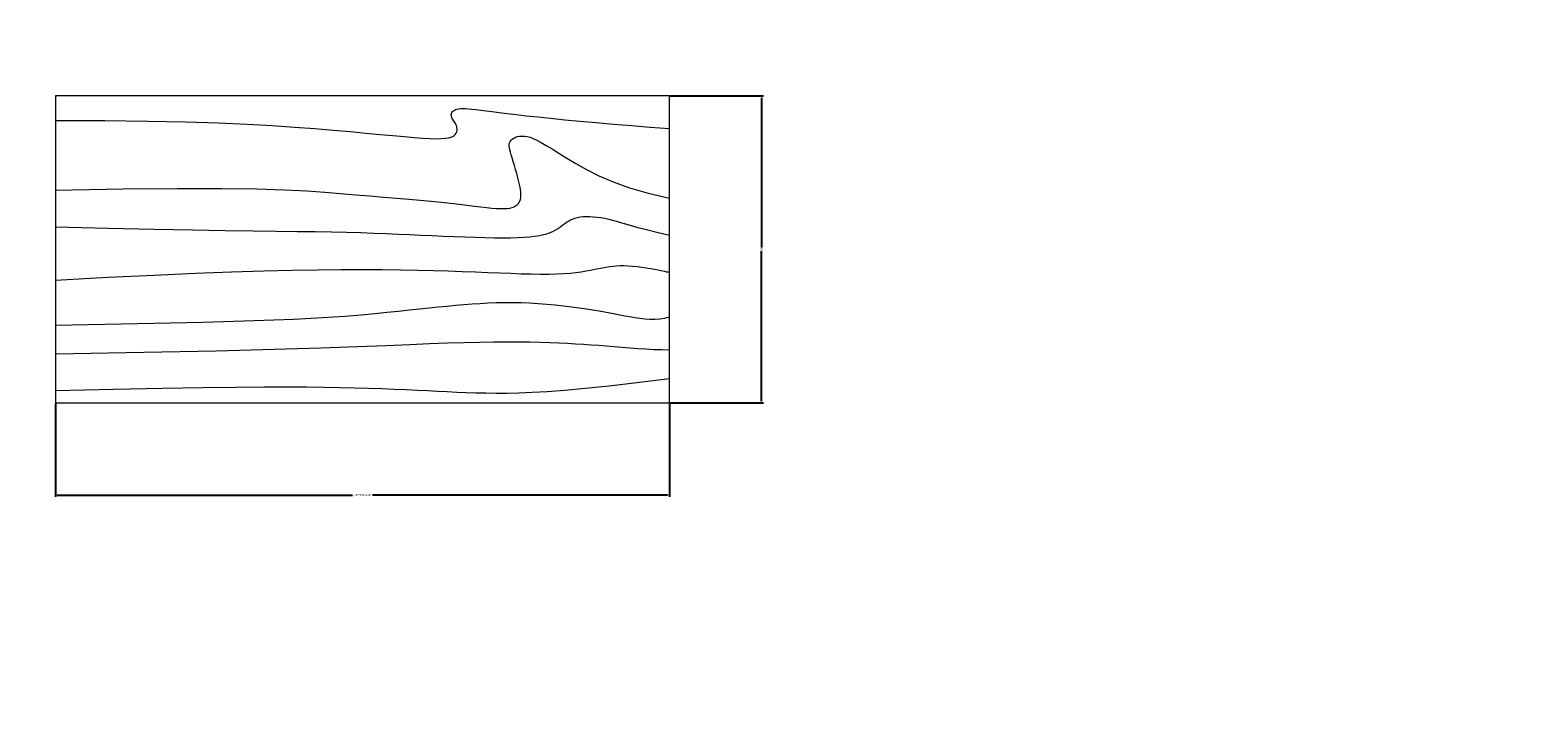
# Model space of a CAD drawing. Units: inches. Extents: x 1563 to 2428, y 777 to 1464.
# Tile 4 of 11: x 1663 to 1810, y 1063 to 1130. Entities that reach past the tile are written whole.
import ezdxf

# ---------------------------------------------------------------- set-up
doc = ezdxf.new("R2010")
doc.units = ezdxf.units.IN
for name, color, linetype, lineweight in [('A-ANNO-DIMS', 2, 'Continuous', 18), ('A-FURN', 9, 'Continuous', 18), ('A-WALL-PATT', 8, 'Continuous', 13)]:
    doc.layers.add(name, color=color, linetype=linetype, lineweight=lineweight)
doc.styles.get("Standard").update_dxf_attribs({"font": 'arial.ttf'})
doc.dimstyles.get("Standard").update_dxf_attribs({"dimtxt": 0.18, "dimasz": 0.18, "dimexe": 0.18, "dimexo": 0.0625, "dimgap": 0.09, "dimtad": 0, "dimtih": 1, "dimtoh": 1, "dimdec": 4, "dimzin": 0, "dimdsep": 46, "dimtxsty": 'Standard', "dimcen": 0.09, "dimadec": 0, "dimazin": 0, "dimtfac": 1, "dimtdec": 4, "dimtofl": 0, "dimtmove": 0, "dimatfit": 3, "dimfxl": 1, "dimtolj": 1, "dimtzin": 0, "dimarcsym": 0})

# ---------------------------------------------------------------- blocks, each defined once
blk = doc.blocks.new('Table - Rectangular Woodgrain 60 x 30 in.')
for p, q in [((0, 0), (0, -30)), ((60, 0), (0, 0)), ((60, -30), (60, 0)), ((0, -30), (60, -30))]:
    blk.add_line(p, q)
for points in [[(0, -2.4), (4.8155, -2.418), (9.0302, -2.4688), (12.709, -2.5477), (15.9167, -2.65), (18.7181, -2.7711), (21.1781, -2.9063), (23.3616, -3.0508), (25.3333, -3.2), (27.1477, -3.3495), (28.8172, -3.4958), (30.3437, -3.636), (31.7291, -3.7667), (32.9756, -3.8849), (34.0849, -3.9875), (35.059, -4.0714), (35.9, -4.1334), (36.6114, -4.1711), (37.2041, -4.1854), (37.6906, -4.1779), (38.0833, -4.15), (38.3948, -4.1034), (38.6375, -4.0396), (38.8239, -3.9602), (38.9666, -3.8667), (39.0764, -3.7608), (39.1573, -3.6448), (39.2116, -3.521), (39.2416, -3.3917), (39.2498, -3.2593), (39.2385, -3.1261), (39.21, -2.9944), (39.1666, -2.8667), (39.111, -2.7447), (39.0468, -2.6281), (38.978, -2.5163), (38.9083, -2.4083), (38.8418, -2.3035), (38.7823, -2.201), (38.7337, -2.1001), (38.7, -2), (38.6844, -1.9003), (38.6875, -1.8021), (38.7094, -1.707), (38.75, -1.6167), (38.8094, -1.5326), (38.8875, -1.4563), (38.9844, -1.3893), (39.1, -1.3333), (39.2351, -1.2896), (39.3937, -1.2583), (39.5804, -1.2396), (39.8, -1.2333), (40.057, -1.2396), (40.3562, -1.2583), (40.7023, -1.2896), (41.1, -1.3333), (41.5547, -1.3895), (42.0755, -1.4573), (42.6721, -1.5361), (43.3542, -1.625), (44.1316, -1.7233), (45.014, -1.8302), (46.0114, -1.9449), (47.1333, -2.0667), (48.3862, -2.1947), (49.7625, -2.3281), (51.2513, -2.4663), (52.8416, -2.6083), (54.5226, -2.7535), (56.2833, -2.9011), (58.1127, -3.0501), (60, -3.2)], [(0, -9.2), (6.5759, -9.0858), (11.9385, -9.0365), (16.2527, -9.0418), (19.6833, -9.0917), (22.3952, -9.1759), (24.5531, -9.2844), (26.322, -9.4069), (27.8666, -9.5333), (29.3241, -9.6553), (30.7203, -9.7719), (32.0532, -9.8837), (33.3208, -9.9917), (34.5213, -10.0965), (35.6526, -10.199), (36.7128, -10.2999), (37.7, -10.4), (38.6129, -10.4996), (39.4531, -10.5969), (40.223, -10.6895), (40.925, -10.775), (41.5613, -10.8512), (42.1344, -10.9156), (42.6465, -10.966), (43.1, -11), (43.4976, -11.0158), (43.8437, -11.0136), (44.143, -10.9942), (44.4, -10.9583), (44.6195, -10.9069), (44.8062, -10.8406), (44.9648, -10.7603), (45.1, -10.6667), (45.2155, -10.5598), (45.3114, -10.4365), (45.3871, -10.2929), (45.4416, -10.125), (45.4743, -9.929), (45.4844, -9.7011), (45.4709, -9.4371), (45.4333, -9.1333), (45.3716, -8.7883), (45.2896, -8.4104), (45.1919, -8.0107), (45.0833, -7.6), (44.9685, -7.1893), (44.8521, -6.7896), (44.7388, -6.4117), (44.6333, -6.0667), (44.54, -5.7628), (44.4614, -5.4979), (44.4001, -5.2675), (44.3583, -5.0667), (44.3384, -4.8909), (44.3427, -4.7354), (44.3736, -4.5956), (44.4333, -4.4667), (44.5236, -4.3453), (44.6427, -4.2333), (44.7884, -4.1339), (44.9583, -4.05), (45.1501, -3.9849), (45.3614, -3.9417), (45.59, -3.9234), (45.8333, -3.9333), (46.0915, -3.9749), (46.3734, -4.0531), (46.6906, -4.1736), (47.0542, -4.3417), (47.4756, -4.5629), (47.9661, -4.8427), (48.5372, -5.1866), (49.2, -5.6), (49.9676, -6.0844), (50.8594, -6.625), (51.8965, -7.2031), (53.1, -7.8), (54.491, -8.3969), (56.0906, -8.975), (57.9199, -9.5156), (60, -10)], [(0, -12.8), (5.1847, -12.9322), (9.6213, -13.0323), (13.3963, -13.1059), (16.5958, -13.1583), (19.3063, -13.1952), (21.614, -13.2219), (23.6054, -13.2439), (25.3666, -13.2667), (26.9728, -13.2947), (28.4531, -13.3281), (29.8256, -13.3663), (31.1083, -13.4083), (32.3191, -13.4535), (33.476, -13.501), (34.597, -13.5501), (35.7, -13.6), (36.7984, -13.6497), (37.8875, -13.6979), (38.9578, -13.743), (40, -13.7833), (41.0047, -13.8174), (41.9625, -13.8438), (42.864, -13.8607), (43.7, -13.8667), (44.4631, -13.8604), (45.1552, -13.8417), (45.7801, -13.8104), (46.3416, -13.7667), (46.8439, -13.7104), (47.2906, -13.6417), (47.6858, -13.5604), (48.0333, -13.4667), (48.3375, -13.3608), (48.6042, -13.2448), (48.8396, -13.121), (49.05, -12.9917), (49.2417, -12.8593), (49.4208, -12.7261), (49.5937, -12.5944), (49.7667, -12.4667), (49.9452, -12.3451), (50.1323, -12.2313), (50.3303, -12.1268), (50.5416, -12.0333), (50.7686, -11.9524), (51.0135, -11.8854), (51.2788, -11.8341), (51.5666, -11.8), (51.8785, -11.7843), (52.2116, -11.7865), (52.562, -11.8059), (52.926, -11.8417), (53.2998, -11.8931), (53.6795, -11.9594), (54.0614, -12.0397), (54.4416, -12.1333), (54.8223, -12.2401), (55.2293, -12.3625), (55.6942, -12.5037), (56.2489, -12.6667), (56.9251, -12.8547), (57.7545, -13.0708), (58.7689, -13.3182), (60, -13.6)], [(0, -18), (5.124, -17.7273), (9.6609, -17.5057), (13.6705, -17.3303), (17.2125, -17.1958), (20.3467, -17.0973), (23.1328, -17.0297), (25.6307, -16.9878), (27.9, -16.9667), (29.9928, -16.9617), (31.9302, -16.9703), (33.7254, -16.9907), (35.3917, -17.0208), (36.9423, -17.0588), (38.3906, -17.1026), (39.7499, -17.1503), (41.0333, -17.2), (42.2519, -17.2496), (43.4073, -17.2969), (44.4986, -17.3395), (45.525, -17.375), (46.4858, -17.4012), (47.3802, -17.4156), (48.2074, -17.416), (48.9667, -17.4), (49.6583, -17.3662), (50.2872, -17.3167), (50.8595, -17.2547), (51.3812, -17.1833), (51.8584, -17.1057), (52.2971, -17.025), (52.7034, -16.9443), (53.0833, -16.8667), (53.443, -16.7951), (53.789, -16.7313), (54.128, -16.6768), (54.4666, -16.6334), (54.8115, -16.6024), (55.1693, -16.5854), (55.5465, -16.5841), (55.95, -16.6), (56.3828, -16.6337), (56.8346, -16.6823), (57.2915, -16.7418), (57.7396, -16.8084), (58.165, -16.878), (58.5539, -16.9469), (58.8924, -17.0111), (59.1666, -17.0667), (59.3679, -17.1107), (59.5078, -17.1438), (59.6032, -17.1675), (59.6708, -17.1833), (59.7275, -17.193), (59.7901, -17.1979), (59.8753, -17.1998), (60, -17.2)], [(0, -22.4), (8.0098, -22.2501), (14.4094, -22.1011), (19.4168, -21.9535), (23.25, -21.8083), (26.1269, -21.6663), (28.2656, -21.5281), (29.884, -21.3947), (31.2, -21.2667), (32.3967, -21.1448), (33.5172, -21.0292), (34.5697, -20.9198), (35.5625, -20.8167), (36.5037, -20.7198), (37.4015, -20.6292), (38.2642, -20.5448), (39.1, -20.4667), (39.9164, -20.3951), (40.7187, -20.3313), (41.5117, -20.2768), (42.3, -20.2333), (43.0883, -20.2024), (43.8812, -20.1854), (44.6836, -20.1841), (45.5, -20.2), (46.3328, -20.234), (47.1747, -20.2844), (48.0163, -20.3488), (48.8479, -20.425), (49.66, -20.5106), (50.4429, -20.6031), (51.1872, -20.7004), (51.8833, -20.8), (52.5246, -20.8999), (53.1166, -20.9995), (53.6681, -21.0983), (54.1875, -21.1958), (54.6834, -21.2919), (55.1646, -21.3859), (55.6394, -21.4777), (56.1167, -21.5667), (56.6028, -21.6515), (57.0961, -21.7266), (57.5929, -21.7852), (58.0896, -21.8208), (58.5823, -21.8268), (59.0674, -21.7964), (59.5412, -21.723), (60, -21.6)], [(0, -25.2), (8.6355, -25.0504), (15.7026, -24.9031), (21.4049, -24.7606), (25.9458, -24.625), (29.529, -24.4988), (32.3578, -24.3844), (34.6359, -24.284), (36.5667, -24.2), (38.3213, -24.1341), (39.9417, -24.0854), (41.437, -24.0523), (42.8167, -24.0333), (44.0901, -24.0268), (45.2667, -24.0313), (46.3557, -24.0451), (47.3667, -24.0667), (48.309, -24.0947), (49.1928, -24.1287), (50.0284, -24.168), (50.826, -24.2125), (51.5959, -24.2617), (52.3483, -24.3151), (53.0935, -24.3725), (53.8417, -24.4334), (54.6009, -24.497), (55.3699, -24.561), (56.1454, -24.6226), (56.9239, -24.6792), (57.7021, -24.7279), (58.4764, -24.7662), (59.2435, -24.7911), (60, -24.8)], [(0, -28.8), (5.6867, -28.6681), (10.45, -28.5698), (14.407, -28.5012), (17.675, -28.4584), (20.3711, -28.4374), (22.6125, -28.4344), (24.5164, -28.4455), (26.2, -28.4667), (27.762, -28.4947), (29.2276, -28.5281), (30.6033, -28.5663), (31.8958, -28.6084), (33.1118, -28.6535), (34.2578, -28.7011), (35.3405, -28.7501), (36.3666, -28.8), (37.3443, -28.8497), (38.288, -28.8974), (39.2137, -28.9412), (40.1375, -28.9792), (41.0753, -29.0093), (42.0432, -29.0297), (43.0572, -29.0384), (44.1333, -29.0333), (45.2936, -29.0114), (46.5843, -28.9641), (48.0579, -28.8816), (49.7666, -28.7542), (51.7629, -28.5721), (54.0989, -28.3255), (56.8272, -28.0048), (60, -27.6)]]:
    blk.add_lwpolyline(points)
blk = doc.blocks.new('*D32')
at = {"layer": 'A-ANNO-DIMS', "color": 0, "lineweight": -2, "transparency": 16777216}
for p, q in [((1664.99, 1093.93), (1664.99, 1084.81)), ((1724.99, 1093.93), (1724.99, 1084.81)), ((1665.17, 1084.99), (1694.02, 1084.99)), ((1724.81, 1084.99), (1695.96, 1084.99))]:
    blk.add_line(p, q, dxfattribs=at)
at = {"layer": 'A-ANNO-DIMS', "color": 0, "transparency": 16777216}
for points in [[(1665.17, 1085.02), (1665.17, 1084.96), (1664.99, 1084.99)], [(1724.81, 1085.02), (1724.81, 1084.96), (1724.99, 1084.99)]]:
    blk.add_solid(points, dxfattribs=at)
at = {"layer": 'Defpoints', "color": 0, "transparency": 16777216}
for p in [(1664.99, 1093.99), (1724.99, 1093.99), (1724.99, 1084.99)]:
    blk.add_point(p, dxfattribs=at)
at = {"layer": 'A-ANNO-DIMS', "color": 0, "transparency": 16777216, "insert": (1694.99, 1084.99), "char_height": 0.18, "attachment_point": 5}
blk.add_mtext('\\A1;LOW TABLE 60', dxfattribs=at)
blk = doc.blocks.new('*D33')
at = {"layer": 'A-ANNO-DIMS', "color": 0, "lineweight": -2, "transparency": 16777216}
for p, q in [((1725.05, 1123.99), (1734.17, 1123.99)), ((1733.99, 1123.81), (1733.99, 1109.17)), ((1733.99, 1094.17), (1733.99, 1108.81)), ((1725.05, 1093.99), (1734.17, 1093.99))]:
    blk.add_line(p, q, dxfattribs=at)
at = {"layer": 'A-ANNO-DIMS', "color": 0, "transparency": 16777216}
for points in [[(1733.96, 1123.81), (1734.02, 1123.81), (1733.99, 1123.99)], [(1733.96, 1094.17), (1734.02, 1094.17), (1733.99, 1093.99)]]:
    blk.add_solid(points, dxfattribs=at)
at = {"layer": 'Defpoints', "color": 0, "transparency": 16777216}
for p in [(1724.99, 1123.99), (1733.99, 1123.99), (1724.99, 1093.99)]:
    blk.add_point(p, dxfattribs=at)
at = {"layer": 'A-ANNO-DIMS', "color": 0, "transparency": 16777216, "insert": (1733.99, 1108.99), "char_height": 0.18, "attachment_point": 5}
blk.add_mtext('\\A1;30', dxfattribs=at)

msp = doc.modelspace()

# ---------------------------------------------------------------- hatches: boundary and pattern name
at = {"layer": 'A-WALL-PATT'}
h = msp.add_hatch(color=256, dxfattribs=at)
h.dxf.hatch_style = 1
h.paths.add_polyline_path([(1965.105, 1421.428), (1605.105, 1421.428), (1605.105, 821.428), (1965.105, 821.428)])
h.paths.add_polyline_path([(1614.105, 1199.428), (1704.105, 1199.428), (1738.605, 1199.428), (1738.605, 1251.928), (1734.105, 1251.928), (1734.105, 1203.928), (1704.105, 1203.928), (1614.105, 1203.928), (1614.105, 1335.928), (1665.105, 1335.928), (1665.105, 1340.428), (1614.105, 1340.428), (1614.105, 1412.428), (1704.105, 1412.428), (1704.105, 1340.428), (1701.105, 1340.428), (1701.105, 1335.928), (1704.105, 1335.928), (1768.605, 1335.928), (1768.605, 1340.428), (1708.605, 1340.428), (1708.605, 1412.428), (1807.605, 1412.428), (1807.605, 1340.428), (1804.605, 1340.428), (1804.605, 1335.928), (1807.605, 1335.928), (1807.605, 1275.928), (1815.105, 1275.928), (1815.105, 1280.428), (1812.105, 1280.428), (1812.105, 1412.428), (1956.105, 1412.428), (1956.105, 1280.428), (1854.105, 1280.428), (1854.105, 1275.928), (1956.105, 1275.928), (1956.105, 830.428), (1614.105, 830.428)], flags=16)
h.paths.add_polyline_path([(1917.224, 1038.928), (1917.224, 1043.846, -0.4014527), (1951.591, 1079.751), (1951.591, 1079.786), (1953.163, 1079.786), (1953.163, 1043.846), (1953.163, 1038.455), (1953.105, 1034.428), (1953.105, 1038.928), (1953.163, 1043.846), (1951.591, 1043.846), (1951.591, 1079.751, 0.4014527), (1917.224, 1043.846), (1917.224, 1038.455), (1917.224, 1034.428), (1834.605, 1034.428), (1834.605, 906.928), (1858.605, 906.928), (1858.605, 954.928), (1932.105, 954.928), (1932.105, 902.428), (1834.605, 902.428), (1834.605, 1034.428), (1914.224, 1034.428), (1914.224, 1038.928)], flags=0)
edge = h.paths.add_edge_path(flags=0)
edge.add_ellipse((1674.345, 1004.483), major_axis=(1.48, 0), ratio=0.8423039, start_angle=90, end_angle=180, ccw=False)
edge.add_line((1674.345, 1005.73), (1674.921, 1005.73))
edge.add_ellipse((2202.617, 985.642), major_axis=(528.234, 0), ratio=0.8423039, start_angle=176.34957, end_angle=177.82005, ccw=False)
edge.add_ellipse((1739.278, 760.804), major_axis=(-313.308, 0), ratio=0.8423039, start_angle=-77.87403, end_angle=-76.21947, ccw=False)
edge.add_ellipse((1739.278, 767.659), major_axis=(305.303, 0), ratio=0.8423039, start_angle=100.20954, end_angle=102.44463, ccw=False)
edge.add_ellipse((1659.357, 1231.328), major_axis=(250.96, 0), ratio=0.8423039, start_angle=-80.74343, end_angle=-77.44507)
edge.add_line((1705.625, 1023.567), (1711.685, 1026.918))
edge.add_ellipse((1711.754, 1026.21), major_axis=(0.74, 0), ratio=0.8423039, start_angle=52.06687, end_angle=90, ccw=False)
edge.add_line((1712.16, 1026.731), (1717.882, 1023.567))
edge.add_ellipse((1764.151, 1231.328), major_axis=(250.96, 0), ratio=0.8423039, start_angle=257.44507, end_angle=260.74343)
edge.add_ellipse((1684.229, 767.659), major_axis=(305.303, 0), ratio=0.8423039, start_angle=77.55537, end_angle=79.79046, ccw=False)
edge.add_ellipse((1684.229, 760.804), major_axis=(-313.308, 0), ratio=0.8423039, start_angle=256.21947, end_angle=257.87403, ccw=False)
edge.add_ellipse((1220.891, 985.642), major_axis=(-528.234, 0), ratio=0.8423039, start_angle=182.17995, end_angle=183.65043, ccw=False)
edge.add_line((1748.586, 1005.73), (1749.162, 1005.73))
edge.add_ellipse((1749.162, 1004.483), major_axis=(-1.48, 0), ratio=0.8423039, start_angle=180, end_angle=270, ccw=False)
edge.add_line((1750.642, 1004.483), (1750.642, 980.28))
edge.add_ellipse((1749.162, 980.28), major_axis=(1.48, 0), ratio=0.8423039, start_angle=270, end_angle=360, ccw=False)
edge.add_ellipse((-8843.864, 962.352), major_axis=(10593.026, 0), ratio=0.84230387, start_angle=-0.3241203, end_angle=0.0902291, ccw=False)
edge.add_ellipse((-8843.864, 962.352), major_axis=(10593.026, 0), ratio=0.84230387, start_angle=-0.3838668, end_angle=-0.3241203, ccw=False)
edge.add_ellipse((1749.162, 890.136), major_axis=(1.48, 0), ratio=0.8423039, start_angle=0, end_angle=90, ccw=False)
edge.add_line((1750.642, 890.136), (1750.642, 865.933))
edge.add_ellipse((1749.162, 865.933), major_axis=(1.48, 0), ratio=0.8423039, start_angle=270, end_angle=360, ccw=False)
edge.add_line((1749.162, 864.686), (1748.528, 864.686))
edge.add_ellipse((-8843.864, 962.352), major_axis=(10593.026, 0), ratio=0.84230387, start_angle=-0.6186432, end_angle=-0.5282715, ccw=False)
edge.add_ellipse((1747.592, 846.206), major_axis=(-2.22, 0), ratio=0.8423039, start_angle=179.37176, end_angle=248.46476, ccw=False)
edge.add_ellipse((-8844.604, 962.352), major_axis=(-10595.313, 0), ratio=0.842303864, start_angle=179.3534459, end_angle=179.3717628, ccw=False)
edge.add_ellipse((1744.512, 842.854), major_axis=(-5.246, 0), ratio=0.8423039, start_angle=90, end_angle=179.35345, ccw=False)
edge.add_line((1744.512, 838.435), (1678.995, 838.435))
edge.add_ellipse((1678.995, 842.854), major_axis=(5.246, 0), ratio=0.8423039, start_angle=180.64655, end_angle=270, ccw=False)
edge.add_ellipse((12268.111, 962.352), major_axis=(-10595.313, 0), ratio=0.84230387, start_angle=0.6282372, end_angle=0.6465541, ccw=False)
edge.add_ellipse((1675.916, 846.206), major_axis=(-2.22, 0), ratio=0.8423039, start_angle=-68.46476, end_angle=0.62824, ccw=False)
edge.add_ellipse((12267.371, 962.352), major_axis=(-10593.026, 0), ratio=0.84230387, start_angle=0.5282715, end_angle=0.6465541, ccw=False)
edge.add_line((1674.98, 864.686), (1674.345, 864.686))
edge.add_ellipse((1674.345, 865.933), major_axis=(-1.48, 0), ratio=0.8423039, start_angle=0, end_angle=90, ccw=False)
edge.add_line((1672.865, 865.933), (1672.865, 890.136))
edge.add_ellipse((1674.345, 890.136), major_axis=(1.48, 0), ratio=0.8423039, start_angle=90, end_angle=180, ccw=False)
edge.add_ellipse((12267.371, 962.352), major_axis=(-10593.026, 0), ratio=0.84230387, start_angle=0.3241203, end_angle=0.3838668, ccw=False)
edge.add_ellipse((12267.371, 962.352), major_axis=(-10593.026, 0), ratio=0.84230387, start_angle=-0.0902291, end_angle=0.3241203, ccw=False)
edge.add_ellipse((1674.345, 980.28), major_axis=(-1.48, 0), ratio=0.8423039, start_angle=0, end_angle=90, ccw=False)
edge.add_line((1672.865, 980.28), (1672.865, 1004.483))
h.paths.add_polyline_path([(1622.542, 1135.584), (1648.534, 1136.233), (1648.683, 1130.234), (1647.126, 1130.196), (1648.323, 1082.21), (1649.88, 1082.249), (1650.03, 1076.251), (1624.038, 1075.603, -0.266667)], flags=0)
edge = h.paths.add_edge_path(flags=0)
edge.add_line((1694.584, 990.705), (1700.334, 994.711))
edge.add_line((1700.334, 994.711), (1702.248, 994.711))
edge.add_line((1702.248, 994.711), (1702.248, 997.061))
edge.add_ellipse((1758.417, 997.061), major_axis=(56.169, 0), ratio=0.8423039, start_angle=150.56143, end_angle=180, ccw=False)
edge.add_ellipse((1665.091, 997.061), major_axis=(-56.169, 0), ratio=0.8423039, start_angle=180, end_angle=209.43857, ccw=False)
edge.add_line((1721.26, 997.061), (1721.26, 994.711))
edge.add_line((1721.26, 994.711), (1723.174, 994.711))
edge.add_line((1723.174, 994.711), (1728.923, 990.705))
edge.add_line((1728.923, 990.705), (1728.923, 975.895))
edge.add_ellipse((1725.091, 976.043), major_axis=(0.357, 6.34), ratio=0.6038336, start_angle=106.34259, end_angle=270.99799, ccw=False)
edge.add_line((1721.26, 975.15), (1721.26, 997.061))
edge.add_ellipse((1665.091, 997.061), major_axis=(-56.169, 0), ratio=0.8423039, start_angle=180, end_angle=209.43857)
edge.add_ellipse((1758.417, 997.061), major_axis=(56.169, 0), ratio=0.8423039, start_angle=150.56143, end_angle=180)
edge.add_line((1702.248, 997.061), (1702.248, 975.15))
edge.add_ellipse((1698.416, 976.043), major_axis=(-0.357, 6.34), ratio=0.6038336, start_angle=89.00201, end_angle=253.65741, ccw=False)
edge.add_line((1694.584, 975.895), (1694.584, 990.705))
edge = h.paths.add_edge_path(flags=0)
edge.add_line((1675.832, 952.075), (1679.883, 938.848))
edge.add_ellipse((5378.107, 931.045), major_axis=(-3698.236, 0), ratio=0.84230387, start_angle=-0.120897, end_angle=0.364076)
edge.add_line((1679.976, 907.545), (1676.149, 892.52))
edge.add_ellipse((12267.371, 962.352), major_axis=(10591.546, 0), ratio=0.84230387, start_angle=180.3241656, end_angle=180.3777642, ccw=False)
edge.add_ellipse((12267.371, 962.352), major_axis=(10591.546, 0), ratio=0.84230387, start_angle=180.0555943, end_angle=180.3241656, ccw=False)
edge = h.paths.add_edge_path(flags=0)
edge.add_ellipse((1706.366, 891.542), major_axis=(81.773, 0), ratio=0.8423039, start_angle=94.27742, end_angle=111.83495, ccw=False)
edge.add_line((1701.225, 960.283), (1722.283, 960.283))
edge.add_ellipse((1717.141, 891.542), major_axis=(-81.773, 0), ratio=0.8423039, start_angle=248.16505, end_angle=265.72258, ccw=False)
edge.add_line((1743.29, 956.803), (1741.105, 940.427))
edge.add_ellipse((1714.553, 877.238), major_axis=(79.58, 0), ratio=0.8423039, start_angle=67.20809, end_angle=85.12993)
edge.add_line((1720.25, 944.097), (1703.258, 944.097))
edge.add_ellipse((1708.954, 877.238), major_axis=(79.58, 0), ratio=0.8423039, start_angle=94.87007, end_angle=112.79191)
edge.add_line((1682.403, 940.427), (1680.218, 956.803))
h.paths.add_polyline_path([(1664.992, 1093.991), (1664.992, 1123.991), (1724.992, 1123.991), (1724.992, 1093.991)], flags=0)
h.paths.add_polyline_path([(1716.588, 1099.729), (1715.404, 1099.805), (1715.021, 1099.823), (1716.177, 1099.758)], flags=0)
h.paths.add_polyline_path([(1711.325, 1103.757), (1712.167, 1103.706), (1713.009, 1103.642), (1713.84, 1103.566), (1715.041, 1103.439), (1716.532, 1103.244), (1717.793, 1103.048), (1718.876, 1102.854), (1719.676, 1102.699), (1720.157, 1102.605), (1720.632, 1102.513), (1721.109, 1102.424), (1721.595, 1102.339), (1722.088, 1102.264), (1722.585, 1102.205), (1723.082, 1102.17), (1723.575, 1102.164), (1724.321, 1102.211), (1724.533, 1102.268), (1723.842, 1102.16), (1722.864, 1102.172), (1721.894, 1102.287), (1720.935, 1102.454), (1720.157, 1102.605), (1719.676, 1102.699), (1719.18, 1102.795), (1718.66, 1102.892), (1718.109, 1102.991), (1717.517, 1103.091), (1716.876, 1103.191), (1716.179, 1103.29), (1715.435, 1103.387), (1714.652, 1103.48), (1713.84, 1103.566), (1713.009, 1103.642), (1712.167, 1103.706), (1711.325, 1103.757), (1710.492, 1103.791), (1709.676, 1103.806), (1708.873, 1103.805), (1707.707, 1103.78), (1707.292, 1103.757), (1708.499, 1103.805), (1710.086, 1103.807)], flags=0)
h.paths.add_polyline_path([(1713.959, 1106.591), (1714.651, 1106.624), (1715.279, 1106.674), (1715.852, 1106.736), (1716.373, 1106.807), (1716.851, 1106.885), (1717.289, 1106.966), (1717.696, 1107.046), (1718.341, 1107.178), (1719.173, 1107.331), (1720.169, 1107.421), (1721.131, 1107.383), (1722.032, 1107.286), (1722.934, 1107.152), (1723.887, 1106.983), (1724.746, 1106.795), (1724.72, 1106.798), (1724.663, 1106.807), (1724.241, 1106.906), (1724.159, 1106.924), (1723.885, 1106.979), (1723.546, 1107.044), (1723.157, 1107.113), (1722.732, 1107.182), (1722.284, 1107.249), (1721.827, 1107.308), (1721.375, 1107.357), (1720.942, 1107.391), (1720.539, 1107.406), (1720.162, 1107.405), (1719.804, 1107.388), (1719.459, 1107.357), (1719.12, 1107.314), (1718.781, 1107.259), (1718.435, 1107.195), (1718.076, 1107.124), (1717.402, 1106.986), (1716.59, 1106.837), (1715.56, 1106.696), (1714.317, 1106.598)], flags=0)
h.paths.add_polyline_path([(1708.692, 1110.124), (1709.455, 1110.13), (1710.147, 1110.149), (1710.772, 1110.18), (1711.334, 1110.224), (1711.836, 1110.28), (1712.283, 1110.349), (1712.678, 1110.43), (1713.026, 1110.524), (1713.33, 1110.63), (1713.596, 1110.746), (1713.832, 1110.87), (1714.042, 1110.999), (1714.234, 1111.131), (1714.413, 1111.264), (1714.586, 1111.396), (1715.065, 1111.75), (1715.879, 1112.11), (1716.842, 1112.224), (1717.903, 1112.165), (1719.048, 1111.965), (1719.867, 1111.736), (1720.686, 1111.487), (1721.596, 1111.22), (1721.917, 1111.136), (1721.028, 1111.383), (1720.222, 1111.628), (1719.815, 1111.75), (1719.434, 1111.857), (1719.054, 1111.951), (1718.672, 1112.031), (1718.292, 1112.097), (1717.918, 1112.149), (1717.554, 1112.185), (1717.204, 1112.204), (1716.871, 1112.206), (1716.559, 1112.191), (1716.271, 1112.156), (1716.006, 1112.105), (1715.761, 1112.038), (1715.534, 1111.957), (1715.323, 1111.864), (1715.125, 1111.759), (1714.937, 1111.645), (1714.759, 1111.524), (1714.586, 1111.396), (1714.413, 1111.264), (1714.003, 1110.96), (1713.331, 1110.606), (1712.501, 1110.382), (1711.61, 1110.245), (1710.489, 1110.158), (1709.111, 1110.121)], flags=0)
h.paths.add_polyline_path([(1707.127, 1113.075), (1707.639, 1113.025), (1708.092, 1112.991), (1708.49, 1112.975), (1708.836, 1112.977), (1709.135, 1112.996), (1709.392, 1113.032), (1709.612, 1113.084), (1709.798, 1113.15), (1709.957, 1113.23), (1710.092, 1113.324), (1710.208, 1113.431), (1710.304, 1113.554), (1710.379, 1113.698), (1710.434, 1113.866), (1710.467, 1114.062), (1710.477, 1114.289), (1710.463, 1114.553), (1710.426, 1114.857), (1710.364, 1115.202), (1710.282, 1115.58), (1710.184, 1115.98), (1710.076, 1116.391), (1709.961, 1116.801), (1709.844, 1117.201), (1709.731, 1117.579), (1709.626, 1117.924), (1709.532, 1118.228), (1709.454, 1118.493), (1709.392, 1118.723), (1709.351, 1118.924), (1709.293, 1119.435), (1709.831, 1119.942), (1710.705, 1120.121), (1711.507, 1119.898), (1712.224, 1119.567), (1713.189, 1119.016), (1713.529, 1118.804), (1712.958, 1119.148), (1712.468, 1119.428), (1712.046, 1119.649), (1711.683, 1119.817), (1711.366, 1119.937), (1711.084, 1120.016), (1710.826, 1120.057), (1710.582, 1120.067), (1710.354, 1120.049), (1710.142, 1120.006), (1709.951, 1119.941), (1709.781, 1119.857), (1709.635, 1119.757), (1709.516, 1119.645), (1709.426, 1119.524), (1709.366, 1119.395), (1709.335, 1119.255), (1709.331, 1119.1), (1709.351, 1118.924), (1709.392, 1118.723), (1709.454, 1118.493), (1709.52, 1118.268), (1709.799, 1117.356), (1710.028, 1116.57), (1710.245, 1115.749), (1710.45, 1114.804), (1710.477, 1114.289), (1710.448, 1113.654), (1709.908, 1113.153), (1709.165, 1112.979), (1708.318, 1112.974), (1707.448, 1113.039)], flags=0)
h.paths.add_polyline_path([(1700.892, 1119.857), (1701.604, 1119.819), (1702.196, 1119.805), (1702.683, 1119.813), (1703.076, 1119.841), (1703.387, 1119.887), (1703.63, 1119.951), (1703.816, 1120.03), (1703.959, 1120.124), (1704.069, 1120.23), (1704.15, 1120.346), (1704.204, 1120.47), (1704.234, 1120.599), (1704.242, 1120.731), (1704.231, 1120.864), (1704.202, 1120.996), (1704.159, 1121.124), (1704.103, 1121.246), (1704.039, 1121.362), (1703.97, 1121.474), (1703.901, 1121.582), (1703.834, 1121.687), (1703.775, 1121.79), (1703.564, 1122.226), (1704.048, 1122.698), (1704.756, 1122.769), (1705.49, 1122.723), (1706.24, 1122.641), (1706.547, 1122.601), (1706.092, 1122.657), (1705.695, 1122.701), (1705.348, 1122.732), (1705.049, 1122.751), (1704.792, 1122.757), (1704.573, 1122.751), (1704.386, 1122.732), (1704.227, 1122.701), (1704.092, 1122.657), (1703.977, 1122.601), (1703.88, 1122.534), (1703.802, 1122.458), (1703.742, 1122.374), (1703.702, 1122.284), (1703.68, 1122.188), (1703.677, 1122.09), (1703.692, 1121.991), (1703.726, 1121.89), (1703.769, 1121.802), (1704.039, 1121.362), (1704.301, 1120.887), (1704.133, 1120.165), (1703.43, 1119.866), (1702.481, 1119.798), (1701.306, 1119.827)], flags=0)
edge = h.paths.add_edge_path(flags=0)
edge.add_ellipse((1711.754, 1009.752), major_axis=(-147.018, 0), ratio=0.8423039, start_angle=76.40187, end_angle=103.59813)
edge.add_line((1741.105, 888.411), (1741.105, 869.587))
edge.add_ellipse((1711.754, 990.928), major_axis=(-147.018, 0), ratio=0.8423039, start_angle=76.40187, end_angle=103.59813, ccw=False)
edge.add_line((1682.403, 869.587), (1682.403, 888.411))
edge = h.paths.add_edge_path(flags=0)
edge.add_ellipse((-8843.864, 962.352), major_axis=(-10591.546, 0), ratio=0.84230387, start_angle=179.6758344, end_angle=179.9444057, ccw=False)
edge.add_ellipse((-8843.864, 962.352), major_axis=(-10591.546, 0), ratio=0.84230387, start_angle=179.6222358, end_angle=179.6758344, ccw=False)
edge.add_line((1747.358, 892.52), (1743.531, 907.545))
edge.add_ellipse((-1954.6, 931.045), major_axis=(3698.236, 0), ratio=0.84230387, start_angle=-0.364076, end_angle=0.120897)
edge.add_line((1743.625, 938.848), (1747.676, 952.075))
h.paths.add_polyline_path([(1637.931, 1162.087), (1637.931, 1188.087, -0.1904762), (1721.931, 1188.087), (1721.931, 1162.087), (1715.931, 1162.087), (1715.931, 1163.644), (1643.931, 1163.644), (1643.931, 1162.087)], flags=0)
h.paths.add_polyline_path([(1667.931, 1189.491, -0.0496282), (1691.931, 1189.491), (1691.931, 1182.705), (1667.931, 1182.705)], flags=0)
edge = h.paths.add_edge_path(flags=0)
edge.add_ellipse((1685.362, 859.825), major_axis=(-2.96, 0), ratio=0.8423039, start_angle=-90, end_angle=0, ccw=False)
edge.add_line((1685.362, 862.318), (1738.145, 862.318))
edge.add_ellipse((1738.145, 859.825), major_axis=(2.96, 0), ratio=0.8423039, start_angle=0, end_angle=90, ccw=False)
edge.add_line((1741.105, 859.825), (1741.105, 840.361))
edge.add_line((1741.105, 840.361), (1682.403, 840.361))
edge.add_line((1682.403, 840.361), (1682.403, 859.825))
h.paths.add_polyline_path([(1777.486, 1164.853), (1777.486, 1180.853), (1778.486, 1181.01), (1778.486, 1164.697)], flags=0)
h.paths.add_polyline_path([(1786.986, 1154.853), (1786.986, 1163.369), (1778.986, 1164.619), (1778.986, 1181.088), (1786.986, 1182.338), (1786.986, 1190.853), (1799.502, 1190.853), (1800.752, 1198.853), (1817.221, 1198.853), (1818.471, 1190.853), (1827.502, 1190.853), (1828.752, 1198.853), (1845.221, 1198.853), (1846.471, 1190.853), (1858.986, 1190.853), (1858.986, 1182.338), (1866.986, 1181.088), (1866.986, 1164.619), (1858.986, 1163.369), (1858.986, 1154.853), (1846.471, 1154.853), (1845.221, 1146.853), (1828.752, 1146.853), (1827.502, 1154.853), (1818.471, 1154.853), (1817.221, 1146.853), (1800.752, 1146.853), (1799.502, 1154.853)], flags=0)
h.paths.add_polyline_path([(1800.986, 1145.353), (1800.83, 1146.353), (1817.143, 1146.353), (1816.986, 1145.353)], flags=0)
h.paths.add_polyline_path([(1851.408, 1167.858), (1852.086, 1167.738), (1852.744, 1167.621), (1853.388, 1167.506), (1854.028, 1167.395), (1854.67, 1167.289), (1855.313, 1167.195), (1855.952, 1167.122), (1856.585, 1167.077), (1857.209, 1167.07), (1858.147, 1167.128), (1858.413, 1167.2), (1857.547, 1167.066), (1856.312, 1167.08), (1855.07, 1167.223), (1854.028, 1167.395), (1853.388, 1167.506), (1852.744, 1167.621), (1852.086, 1167.738), (1851.408, 1167.858), (1850.288, 1168.052), (1849.956, 1168.104), (1850.701, 1167.98)], flags=0)
h.paths.add_polyline_path([(1845.435, 1172.646), (1846.222, 1172.707), (1846.941, 1172.785), (1847.601, 1172.874), (1848.21, 1172.971), (1848.777, 1173.072), (1849.311, 1173.173), (1850.14, 1173.331), (1851.063, 1173.483), (1852.014, 1173.591), (1853.012, 1173.633), (1854.075, 1173.594), (1855.251, 1173.473), (1856.4, 1173.306), (1857.391, 1173.132), (1857.945, 1173.02), (1858.196, 1172.965), (1858.595, 1172.871), (1858.575, 1172.874), (1858.49, 1172.894), (1858.371, 1172.924), (1858.196, 1172.965), (1857.945, 1173.02), (1857.602, 1173.089), (1857.177, 1173.17), (1856.687, 1173.256), (1856.148, 1173.343), (1855.575, 1173.426), (1854.986, 1173.5), (1854.395, 1173.561), (1853.82, 1173.603), (1853.272, 1173.623), (1852.749, 1173.622), (1852.247, 1173.6), (1851.757, 1173.562), (1851.276, 1173.507), (1850.796, 1173.439), (1850.313, 1173.359), (1849.82, 1173.27), (1849.311, 1173.173), (1848.421, 1173.005), (1847.25, 1172.818), (1845.826, 1172.665)], flags=0)
h.paths.add_polyline_path([(1840.587, 1177.09), (1841.289, 1177.145), (1841.916, 1177.215), (1842.475, 1177.301), (1842.969, 1177.403), (1843.403, 1177.52), (1843.783, 1177.652), (1844.117, 1177.797), (1844.411, 1177.952), (1844.674, 1178.114), (1844.914, 1178.279), (1845.138, 1178.446), (1845.644, 1178.831), (1846.285, 1179.221), (1847.125, 1179.521), (1847.998, 1179.624), (1848.834, 1179.619), (1849.768, 1179.529), (1850.775, 1179.363), (1851.78, 1179.14), (1852.111, 1179.053), (1851.57, 1179.187), (1851.043, 1179.304), (1850.527, 1179.404), (1850.024, 1179.487), (1849.539, 1179.551), (1849.072, 1179.596), (1848.628, 1179.62), (1848.21, 1179.623), (1847.82, 1179.603), (1847.46, 1179.561), (1847.128, 1179.497), (1846.822, 1179.413), (1846.539, 1179.312), (1846.274, 1179.195), (1846.027, 1179.064), (1845.793, 1178.922), (1845.57, 1178.77), (1845.354, 1178.61), (1844.817, 1178.201), (1844.106, 1177.764), (1843.208, 1177.452), (1842.225, 1177.25), (1840.973, 1177.11)], flags=0)
h.paths.add_polyline_path([(1836.67, 1180.646), (1837.236, 1180.603), (1837.734, 1180.584), (1838.166, 1180.586), (1838.54, 1180.611), (1838.861, 1180.655), (1839.136, 1180.72), (1839.369, 1180.803), (1839.568, 1180.903), (1839.736, 1181.02), (1839.881, 1181.152), (1840.001, 1181.299), (1840.095, 1181.456), (1840.164, 1181.624), (1840.204, 1181.8), (1840.217, 1181.981), (1840.2, 1182.166), (1840.153, 1182.353), (1840.076, 1182.541), (1839.973, 1182.728), (1839.851, 1182.916), (1839.716, 1183.103), (1839.572, 1183.291), (1839.427, 1183.478), (1839.033, 1184), (1838.862, 1184.411), (1838.695, 1184.99), (1839.2, 1185.669), (1840.06, 1185.961), (1840.793, 1185.931), (1841.454, 1185.77), (1842.179, 1185.536), (1842.706, 1185.363), (1843.713, 1185.044), (1844.033, 1184.956), (1843.102, 1185.234), (1842.179, 1185.536), (1841.725, 1185.682), (1841.328, 1185.801), (1840.976, 1185.886), (1840.653, 1185.937), (1840.349, 1185.949), (1840.063, 1185.926), (1839.799, 1185.872), (1839.559, 1185.791), (1839.347, 1185.686), (1839.165, 1185.562), (1839.016, 1185.422), (1838.903, 1185.27), (1838.828, 1185.11), (1838.79, 1184.943), (1838.784, 1184.77), (1838.809, 1184.593), (1838.862, 1184.411), (1838.938, 1184.227), (1839.036, 1184.041), (1839.153, 1183.853), (1839.285, 1183.666), (1839.427, 1183.478), (1839.572, 1183.291), (1839.716, 1183.103), (1839.851, 1182.916), (1840.178, 1182.415), (1840.251, 1181.604), (1839.686, 1180.915), (1838.893, 1180.633), (1837.976, 1180.574), (1837.01, 1180.612)], flags=0)
h.paths.add_polyline_path([(1829.867, 1185.622), (1830.475, 1185.631), (1830.966, 1185.666), (1831.355, 1185.724), (1831.658, 1185.804), (1831.891, 1185.903), (1832.07, 1186.02), (1832.207, 1186.152), (1832.308, 1186.297), (1832.376, 1186.452), (1832.414, 1186.614), (1832.424, 1186.779), (1832.41, 1186.946), (1832.374, 1187.11), (1832.32, 1187.27), (1832.25, 1187.422), (1832.17, 1187.568), (1832.084, 1187.708), (1831.997, 1187.843), (1831.914, 1187.974), (1831.839, 1188.102), (1831.614, 1188.57), (1832.036, 1189.169), (1832.801, 1189.319), (1833.589, 1189.3), (1834.44, 1189.223), (1834.736, 1189.187), (1834.239, 1189.241), (1833.807, 1189.28), (1833.433, 1189.304), (1833.111, 1189.312), (1832.837, 1189.304), (1832.604, 1189.28), (1832.405, 1189.241), (1832.236, 1189.187), (1832.092, 1189.117), (1831.971, 1189.033), (1831.873, 1188.938), (1831.799, 1188.832), (1831.748, 1188.719), (1831.721, 1188.601), (1831.717, 1188.478), (1831.736, 1188.353), (1831.779, 1188.228), (1831.839, 1188.102), (1831.914, 1187.974), (1831.997, 1187.843), (1832.084, 1187.708), (1832.387, 1187.216), (1832.456, 1186.393), (1831.916, 1185.871), (1831.195, 1185.682), (1830.221, 1185.613)], flags=0)
h.paths.add_polyline_path([(1828.986, 1145.353), (1828.83, 1146.353), (1845.143, 1146.353), (1844.986, 1145.353)], flags=0)
h.paths.add_polyline_path([(1800.986, 1200.353), (1816.986, 1200.353), (1817.143, 1199.353), (1800.83, 1199.353)], flags=0)
h.paths.add_polyline_path([(1828.986, 1200.353), (1844.986, 1200.353), (1845.143, 1199.353), (1828.83, 1199.353)], flags=0)
h.paths.add_polyline_path([(1867.486, 1181.01), (1868.486, 1180.853), (1868.486, 1164.853), (1867.486, 1164.697)], flags=0)
h.paths.add_polyline_path([(1901.055, 1112.089), (1901.055, 1241.889), (1954.299, 1241.889), (1954.299, 1112.089)], flags=0)
h.paths.add_polyline_path([(1908.544, 1229.408), (1931.009, 1229.408), (1937.23, 1216.927), (1931.009, 1216.927), (1931.009, 1129.562), (1908.544, 1129.562)], flags=0)
h.paths.add_polyline_path([(1699.472, 1381.538), (1701.045, 1381.538), (1701.045, 1345.599), (1699.472, 1345.599)], flags=0)
h.paths.add_polyline_path([(1851.045, 1285.819), (1851.045, 1280.428), (1851.105, 1275.928), (1851.105, 1280.428)], flags=0)
h.paths.add_polyline_path([(1815.105, 1285.819), (1815.105, 1321.758), (1816.678, 1321.758), (1816.678, 1285.819)], flags=0)
h.paths.add_polyline_path([(1745.154, 1343.707, -0.1044693), (1742.568, 1347.148, -0.1176343), (1741.799, 1350.905, -0.1176343), (1742.808, 1354.603, -0.1044693), (1745.61, 1357.871, -0.0900158), (1749.544, 1359.891, -0.0819199), (1754.355, 1360.526, -0.0819199), (1759.115, 1359.583, -0.0900158), (1762.911, 1357.314, -0.1044693), (1765.497, 1353.872, -0.1176343), (1766.266, 1350.116, -0.1176343), (1765.257, 1346.417, -0.1044693), (1762.455, 1343.149, -0.0900158), (1758.521, 1341.13, -0.0819199), (1753.71, 1340.495, -0.0819199), (1748.95, 1341.438, -0.0900158)], flags=0)
h.paths.add_polyline_path([(1745.961, 1344.152, -0.1046782), (1743.517, 1347.257, -0.1186217), (1742.746, 1350.669, -0.1186217), (1743.612, 1354.059, -0.1046782), (1746.143, 1357.094, -0.0895621), (1749.732, 1359.002, -0.0811847), (1754.161, 1359.662, -0.0811847), (1758.57, 1358.877, -0.0895621), (1762.104, 1356.869, -0.1046782), (1764.548, 1353.764, -0.1186217), (1765.319, 1350.351, -0.1186217), (1764.453, 1346.962, -0.1046782), (1761.922, 1343.927, -0.0895621), (1758.333, 1342.019, -0.0811847), (1753.904, 1341.359, -0.0811847), (1749.495, 1342.143, -0.0895621)], flags=0)
h.paths.add_polyline_path([(1748.738, 1346.3, -0.1046075), (1747.125, 1348.343, -0.1182826), (1746.612, 1350.593, -0.1182826), (1747.176, 1352.832, -0.1046075), (1748.833, 1354.838, -0.089718), (1751.19, 1356.103, -0.0814361), (1754.1, 1356.547, -0.0814361), (1756.999, 1356.038, -0.089718), (1759.327, 1354.72, -0.1046075), (1760.94, 1352.678, -0.1182826), (1761.453, 1350.427, -0.1182826), (1760.889, 1348.189, -0.1046075), (1759.232, 1346.183, -0.089718), (1756.875, 1344.917, -0.0814361), (1753.965, 1344.474, -0.0814361), (1751.066, 1344.982, -0.089718)], flags=0)
h.paths.add_polyline_path([(1802.972, 1381.538), (1804.545, 1381.538), (1804.545, 1345.599), (1802.972, 1345.599)], flags=0)
h.paths.add_polyline_path([(1752.533, 1350.51, -1), (1755.533, 1350.51, -1)], flags=0)
h.paths.add_polyline_path([(1753.033, 1350.51, -1), (1755.033, 1350.51, -1)], flags=0)
h.paths.add_polyline_path([(1869.759, 1336.236), (1869.759, 1396.236), (1949.759, 1396.236), (1949.759, 1336.236)], flags=0)
h.paths.add_polyline_path([(1920.159, 1336.236), (1920.159, 1351.436), (1935.359, 1351.436), (1935.359, 1388.236), (1948.559, 1388.236), (1948.559, 1367.436), (1935.359, 1367.436), (1935.359, 1365.036), (1948.559, 1365.036), (1948.559, 1344.236), (1933.359, 1344.236), (1933.359, 1349.436)], flags=0)
h.paths.add_polyline_path([(1938.156, 1328.719, -1), (1952.156, 1328.719, -1)], flags=0)
h.paths.add_polyline_path([(1942.156, 1328.719), (1945.156, 1331.719), (1948.156, 1328.719), (1945.156, 1325.719)], flags=0)
h.paths.add_polyline_path([(1944.156, 1328.719, -1), (1946.156, 1328.719, -1)], flags=0)
h.paths.add_polyline_path([(1914.224, 1038.928), (1614.105, 1038.928), (1614.105, 1034.428), (1830.105, 1034.428), (1830.105, 830.428), (1834.605, 830.428), (1834.605, 1034.428), (1914.224, 1034.428)], flags=0)
h.paths.add_polyline_path([(1956.105, 902.428), (1834.605, 902.428), (1834.605, 830.428), (1956.105, 830.428)], flags=0)

# ---------------------------------------------------------------- block references
at = {"layer": 'A-FURN'}
msp.add_blockref('Table - Rectangular Woodgrain 60 x 30 in.', (1664.992, 1123.991), dxfattribs=at)

# ---------------------------------------------------------------- dimensions: what is measured, and where the dimension line sits
at = {"layer": 'A-ANNO-DIMS'}
dim = msp.add_linear_dim(base=(1733.992, 1123.991), p1=(1724.992, 1093.991), p2=(1724.992, 1123.991), angle=90, dimstyle='Standard', override={"dimdec": 0, "dimlfac": 1, "dimrnd": 0, "dimzin": 0, "dimdsep": 46, "dimlunit": 2}, dxfattribs=at)
dim.commit()
dim.dimension.update_dxf_attribs({"geometry": '*D33', "text_midpoint": (1733.992, 1108.991)})
dim = msp.add_linear_dim(base=(1724.992, 1084.991), p1=(1664.992, 1093.991), p2=(1724.992, 1093.991), text='LOW TABLE <>', dimstyle='Standard', override={"dimdec": 0, "dimlfac": 1, "dimrnd": 0, "dimzin": 0, "dimdsep": 46, "dimlunit": 2}, dxfattribs=at)
dim.commit()
dim.dimension.update_dxf_attribs({"geometry": '*D32', "text_midpoint": (1694.992, 1084.991)})

doc.saveas('drawing.dxf')
